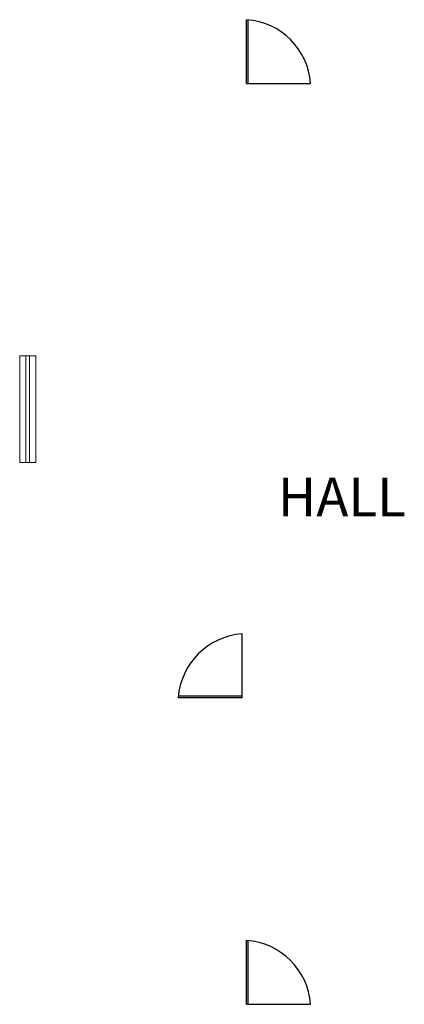
# Model space of a CAD drawing. Units: inches. Extents: x -335 to 1312, y -66 to 821.
# Tile 1 of 4: x -335 to -119, y 104 to 658. Entities that reach past the tile are written whole.
import ezdxf

# ---------------------------------------------------------------- set-up
doc = ezdxf.new("R2010")
doc.units = ezdxf.units.IN
doc.header["$MEASUREMENT"] = 0
for name, color, linetype, lineweight in [('A-AREA-IDEN', 7, 'Continuous', 25), ('A-DOOR', 34, 'Continuous', 25), ('A-GLAZ', 34, 'Continuous', 18)]:
    doc.layers.add(name, color=color, linetype=linetype, lineweight=lineweight)
doc.styles.get("Standard").update_dxf_attribs({"font": 'arial.ttf'})

# ---------------------------------------------------------------- blocks, each defined once
blk = doc.blocks.new('WIN-60IN')
for p, q in [((9, 60), (0, 60)), ((0, 60), (0, 0)), ((3.5, 60), (3.5, 0)), ((5.5, 60), (5.5, 0)), ((9, 0), (9, 60)), ((0, 0), (9, 0))]:
    blk.add_line(p, q)
blk = doc.blocks.new('DOOR-SWING-36IN')
for p, q in [((0, 0), (0, 35.94)), ((1, 0), (1, 35.86)), ((0, 0), (36, 0))]:
    blk.add_line(p, q)
blk.add_arc((-2.68, -2.74), 38.78, 4.0546, 86.0352)

msp = doc.modelspace()

# ---------------------------------------------------------------- block references
at = {"layer": 'A-DOOR'}
for p in [(-207.74, 622.35), (-207.74, 103.9)]:
    msp.add_blockref('DOOR-SWING-36IN', p, dxfattribs=at)
at = {"layer": 'A-DOOR', "rotation": 89.99999999999947}
msp.add_blockref('DOOR-SWING-36IN', (-210.2, 276.48), dxfattribs=at)
at = {"layer": 'A-GLAZ'}
msp.add_blockref('WIN-60IN', (-335.31, 408.95), dxfattribs=at)

# ---------------------------------------------------------------- texts
at = {"layer": 'A-AREA-IDEN'}
msp.add_text('HALL', height=21.784, dxfattribs=at).set_placement((-190.14, 378.58))

doc.saveas('drawing.dxf')
